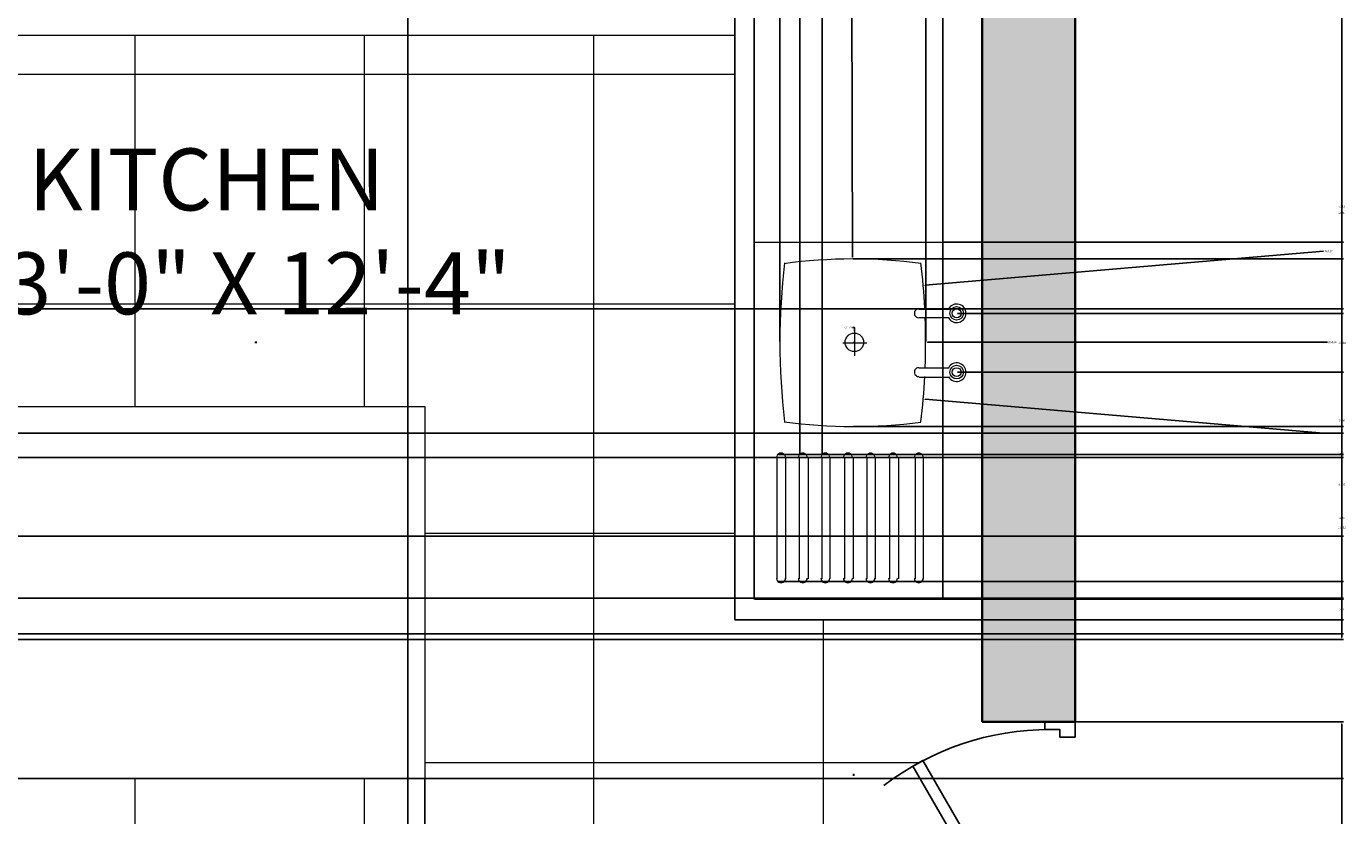
# Model space of a CAD drawing. Units: inches. Extents: x 6 to 575, y 34 to 566.
# Tile 20 of 21: x 447 to 575, y 432 to 508. Entities that reach past the tile are written whole.
import ezdxf

# ---------------------------------------------------------------- set-up
doc = ezdxf.new("R2010")
doc.units = ezdxf.units.IN
for name, color, linetype, lineweight in [('A-ANNO-DIMS', 2, 'Continuous', 18), ('A-AREA-IDEN', 6, 'Continuous', 20), ('A-FLOR-CASE', 2, 'Continuous', 18), ('A-FLOR-FIXT', 9, 'Continuous', 18), ('A-FLOR-PATT', 252, 'Continuous', 9), ('A-WALL-PATT', 251, 'Continuous', 9), ('DOORS', 3, 'Continuous', 25), ('WALLS', 7, 'Continuous', 35)]:
    doc.layers.add(name, color=color, linetype=linetype, lineweight=lineweight)
doc.styles.add('PDF Arial Narrow', font='txt')
doc.styles.get("Standard").update_dxf_attribs({"font": 'arial.ttf'})
doc.dimstyles.get("Standard").update_dxf_attribs({"dimtxt": 0.18, "dimasz": 0.18, "dimexe": 0.18, "dimexo": 0.0625, "dimgap": 0.09, "dimtad": 0, "dimtih": 1, "dimtoh": 1, "dimdec": 4, "dimzin": 0, "dimdsep": 46, "dimtxsty": 'Standard', "dimcen": 0.09, "dimadec": 0, "dimazin": 0, "dimtfac": 1, "dimtdec": 4, "dimtofl": 0, "dimtmove": 0, "dimatfit": 3, "dimfxl": 1, "dimtolj": 1, "dimtzin": 0, "dimarcsym": 0})

# ---------------------------------------------------------------- blocks, each defined once
blk = doc.blocks.new('Door - Left Hung 36 in.')
blk.add_lwpolyline([(0.75, -1.3), (0, 0), (31.18, 18), (31.93, 16.7)], close=True)
blk.add_arc((0, 0), 36, 0, 37.3101)
blk = doc.blocks.new('*D47')
at = {"layer": 'A-ANNO-DIMS', "color": 0, "lineweight": -2, "transparency": 16777216}
for p, q in [((548.72, 440.8), (574.68, 440.8)), ((574.5, 440.62), (574.5, 426.98)), ((574.5, 412.98), (574.5, 426.62)), ((548.72, 412.8), (574.68, 412.8))]:
    blk.add_line(p, q, dxfattribs=at)
at = {"layer": 'A-ANNO-DIMS', "color": 0, "transparency": 16777216}
for points in [[(574.47, 440.62), (574.53, 440.62), (574.5, 440.8)], [(574.47, 412.98), (574.53, 412.98), (574.5, 412.8)]]:
    blk.add_solid(points, dxfattribs=at)
at = {"layer": 'Defpoints', "color": 0, "transparency": 16777216}
for p in [(548.66, 440.8), (574.5, 440.8), (548.66, 412.8)]:
    blk.add_point(p, dxfattribs=at)
at = {"layer": 'A-ANNO-DIMS', "color": 0, "transparency": 16777216, "insert": (574.5, 426.8), "char_height": 0.18, "attachment_point": 5}
blk.add_mtext('\\A1;28', dxfattribs=at)
blk = doc.blocks.new('*D50')
at = {"layer": 'A-ANNO-DIMS', "color": 0, "lineweight": -2, "transparency": 16777216}
for p, q in [((248.7, 468.78), (574.68, 468.78)), ((574.5, 468.6), (574.5, 463.96)), ((574.5, 458.97), (574.5, 463.6)), ((248.7, 458.79), (574.68, 458.79))]:
    blk.add_line(p, q, dxfattribs=at)
at = {"layer": 'A-ANNO-DIMS', "color": 0, "transparency": 16777216}
for points in [[(574.47, 468.6), (574.53, 468.6), (574.5, 468.78)], [(574.47, 458.97), (574.53, 458.97), (574.5, 458.79)]]:
    blk.add_solid(points, dxfattribs=at)
at = {"layer": 'Defpoints', "color": 0, "transparency": 16777216}
for p in [(248.63, 468.78), (574.5, 468.78), (248.63, 458.79)]:
    blk.add_point(p, dxfattribs=at)
at = {"layer": 'A-ANNO-DIMS', "color": 0, "transparency": 16777216, "insert": (574.5, 463.78), "char_height": 0.18, "attachment_point": 5}
blk.add_mtext('\\A1;9.987', dxfattribs=at)
blk = doc.blocks.new('*D51')
at = {"layer": 'A-ANNO-DIMS', "color": 0, "lineweight": -2, "transparency": 16777216}
for p, q in [((437.69, 435.25), (437.69, 33.76)), ((485.67, 435.25), (485.67, 33.76)), ((437.87, 33.94), (461.28, 33.94)), ((485.49, 33.94), (462.08, 33.94))]:
    blk.add_line(p, q, dxfattribs=at)
at = {"layer": 'A-ANNO-DIMS', "color": 0, "transparency": 16777216}
for points in [[(437.87, 33.97), (437.87, 33.91), (437.69, 33.94)], [(485.49, 33.97), (485.49, 33.91), (485.67, 33.94)]]:
    blk.add_solid(points, dxfattribs=at)
at = {"layer": 'Defpoints', "color": 0, "transparency": 16777216}
for p in [(437.69, 435.31), (485.67, 435.31), (485.67, 33.94)]:
    blk.add_point(p, dxfattribs=at)
at = {"layer": 'A-ANNO-DIMS', "color": 0, "transparency": 16777216, "insert": (461.68, 33.94), "char_height": 0.18, "attachment_point": 5}
blk.add_mtext('\\A1;47.98', dxfattribs=at)
blk = doc.blocks.new('*D53')
at = {"layer": 'A-ANNO-DIMS', "color": 0, "lineweight": -2, "transparency": 16777216}
for p, q in [((445.02, 338), (445.02, 565.81)), ((445.2, 565.63), (464.15, 565.63)), ((483.85, 565.63), (464.9, 565.63)), ((484.03, 338), (484.03, 565.81))]:
    blk.add_line(p, q, dxfattribs=at)
at = {"layer": 'A-ANNO-DIMS', "color": 0, "transparency": 16777216}
for points in [[(445.2, 565.66), (445.2, 565.6), (445.02, 565.63)], [(483.85, 565.66), (483.85, 565.6), (484.03, 565.63)]]:
    blk.add_solid(points, dxfattribs=at)
at = {"layer": 'Defpoints', "color": 0, "transparency": 16777216}
for p in [(484.03, 565.63), (445.02, 337.94), (484.03, 337.94)]:
    blk.add_point(p, dxfattribs=at)
at = {"layer": 'A-ANNO-DIMS', "color": 0, "transparency": 16777216, "insert": (464.53, 565.63), "char_height": 0.18, "attachment_point": 5}
blk.add_mtext('\\A1;39.01', dxfattribs=at)
blk = doc.blocks.new('*D64')
at = {"layer": 'A-ANNO-DIMS', "color": 0, "lineweight": -2, "transparency": 16777216}
for p, q in [((354.721145, 452.800984), (574.675816, 452.800984)), ((574.495816, 452.620984), (574.495816, 450.980984)), ((574.495816, 448.980984), (574.495816, 450.620984)), ((354.721145, 448.800984), (574.675816, 448.800984))]:
    blk.add_line(p, q, dxfattribs=at)
at = {"layer": 'A-ANNO-DIMS', "color": 0, "transparency": 16777216}
for points in [[(574.465816, 452.620984), (574.525816, 452.620984), (574.495816, 452.800984)], [(574.465816, 448.980984), (574.525816, 448.980984), (574.495816, 448.800984)]]:
    blk.add_solid(points, dxfattribs=at)
at = {"layer": 'Defpoints', "color": 0, "transparency": 16777216}
for p in [(354.658645, 452.800984), (574.495816, 452.800984), (354.658645, 448.800984)]:
    blk.add_point(p, dxfattribs=at)
at = {"layer": 'A-ANNO-DIMS', "color": 0, "transparency": 16777216, "insert": (574.495816, 450.800984), "char_height": 0.18, "attachment_point": 5}
blk.add_mtext('\\A1;4', dxfattribs=at)
blk = doc.blocks.new('*D151')
at = {"layer": 'A-ANNO-DIMS', "color": 0, "lineweight": -2, "transparency": 16777216}
for p, q in [((437.75, 435.31), (574.68, 435.31)), ((574.5, 435.13), (574.5, 421.25)), ((574.5, 407.01), (574.5, 420.89)), ((433.77, 406.83), (574.68, 406.83))]:
    blk.add_line(p, q, dxfattribs=at)
at = {"layer": 'A-ANNO-DIMS', "color": 0, "transparency": 16777216}
for points in [[(574.47, 435.13), (574.53, 435.13), (574.5, 435.31)], [(574.47, 407.01), (574.53, 407.01), (574.5, 406.83)]]:
    blk.add_solid(points, dxfattribs=at)
at = {"layer": 'Defpoints', "color": 0, "transparency": 16777216}
for p in [(437.69, 435.31), (433.71, 406.83), (574.5, 406.83)]:
    blk.add_point(p, dxfattribs=at)
at = {"layer": 'A-ANNO-DIMS', "color": 0, "transparency": 16777216, "insert": (574.5, 421.07), "char_height": 0.18, "attachment_point": 5}
blk.add_mtext('\\A1;28.48', dxfattribs=at)
blk = doc.blocks.new('*D152')
at = {"layer": 'A-ANNO-DIMS', "color": 0, "lineweight": -2, "transparency": 16777216}
for p, q in [((383.72, 530.8), (574.68, 530.8)), ((574.5, 530.62), (574.5, 490.26)), ((574.5, 449.53), (574.5, 489.89)), ((383.72, 449.35), (574.68, 449.35))]:
    blk.add_line(p, q, dxfattribs=at)
at = {"layer": 'A-ANNO-DIMS', "color": 0, "transparency": 16777216}
for points in [[(574.47, 530.62), (574.53, 530.62), (574.5, 530.8)], [(574.47, 449.53), (574.53, 449.53), (574.5, 449.35)]]:
    blk.add_solid(points, dxfattribs=at)
at = {"layer": 'Defpoints', "color": 0, "transparency": 16777216}
for p in [(383.66, 530.8), (574.5, 530.8), (383.66, 449.35)]:
    blk.add_point(p, dxfattribs=at)
at = {"layer": 'A-ANNO-DIMS', "color": 0, "transparency": 16777216, "insert": (574.5, 490.08), "char_height": 0.18, "attachment_point": 5}
blk.add_mtext('\\A1;81.45', dxfattribs=at)
blk = doc.blocks.new('*D153')
at = {"layer": 'A-ANNO-DIMS', "color": 0, "lineweight": -2, "transparency": 16777216}
for p, q in [((539.72, 530.8), (574.68, 530.8)), ((574.5, 530.62), (574.5, 490.92)), ((574.5, 450.86), (574.5, 490.56)), ((539.72, 450.68), (574.68, 450.68))]:
    blk.add_line(p, q, dxfattribs=at)
at = {"layer": 'A-ANNO-DIMS', "color": 0, "transparency": 16777216}
for points in [[(574.47, 530.62), (574.53, 530.62), (574.5, 530.8)], [(574.47, 450.86), (574.53, 450.86), (574.5, 450.68)]]:
    blk.add_solid(points, dxfattribs=at)
at = {"layer": 'Defpoints', "color": 0, "transparency": 16777216}
for p in [(539.66, 530.8), (574.5, 530.8), (539.66, 450.68)]:
    blk.add_point(p, dxfattribs=at)
at = {"layer": 'A-ANNO-DIMS', "color": 0, "transparency": 16777216, "insert": (574.5, 490.74), "char_height": 0.18, "attachment_point": 5}
blk.add_mtext('\\A1;80.12', dxfattribs=at)
blk = doc.blocks.new('*D155')
at = {"layer": 'A-ANNO-DIMS', "color": 0, "lineweight": -2, "transparency": 16777216}
for p, q in [((515.71, 450.74), (515.71, 565.81)), ((515.89, 565.63), (516.33, 565.63)), ((517.4, 565.63), (516.96, 565.63)), ((517.58, 452.77), (517.58, 565.81))]:
    blk.add_line(p, q, dxfattribs=at)
at = {"layer": 'A-ANNO-DIMS', "color": 0, "transparency": 16777216}
for points in [[(515.89, 565.66), (515.89, 565.6), (515.71, 565.63)], [(517.4, 565.66), (517.4, 565.6), (517.58, 565.63)]]:
    blk.add_solid(points, dxfattribs=at)
at = {"layer": 'Defpoints', "color": 0, "transparency": 16777216}
for p in [(517.58, 565.63), (517.58, 452.71), (515.71, 450.68)]:
    blk.add_point(p, dxfattribs=at)
at = {"layer": 'A-ANNO-DIMS', "color": 0, "transparency": 16777216, "insert": (516.64, 565.63), "char_height": 0.18, "attachment_point": 5}
blk.add_mtext('\\A1;1.87', dxfattribs=at)
blk = doc.blocks.new('*D156')
at = {"layer": 'A-ANNO-DIMS', "color": 0, "lineweight": -2, "transparency": 16777216}
for p, q in [((535.9, 487.27), (574.68, 487.27)), ((574.5, 487.09), (574.5, 470.17)), ((574.5, 452.89), (574.5, 469.81)), ((517.64, 452.71), (574.68, 452.71))]:
    blk.add_line(p, q, dxfattribs=at)
at = {"layer": 'A-ANNO-DIMS', "color": 0, "transparency": 16777216}
for points in [[(574.47, 487.09), (574.53, 487.09), (574.5, 487.27)], [(574.47, 452.89), (574.53, 452.89), (574.5, 452.71)]]:
    blk.add_solid(points, dxfattribs=at)
at = {"layer": 'Defpoints', "color": 0, "transparency": 16777216}
for p in [(535.84, 487.27), (574.5, 487.27), (517.58, 452.71)]:
    blk.add_point(p, dxfattribs=at)
at = {"layer": 'A-ANNO-DIMS', "color": 0, "transparency": 16777216, "insert": (574.5, 469.99), "char_height": 0.18, "attachment_point": 5}
blk.add_mtext('\\A1;34.56', dxfattribs=at)
blk = doc.blocks.new('*D157')
at = {"layer": 'A-ANNO-DIMS', "color": 0, "lineweight": -2, "transparency": 16777216}
for p, q in [((517.58, 452.77), (517.58, 565.81)), ((517.76, 565.63), (526.25, 565.63)), ((535.66, 565.63), (527.16, 565.63)), ((535.84, 452.77), (535.84, 565.81))]:
    blk.add_line(p, q, dxfattribs=at)
at = {"layer": 'A-ANNO-DIMS', "color": 0, "transparency": 16777216}
for points in [[(517.76, 565.66), (517.76, 565.6), (517.58, 565.63)], [(535.66, 565.66), (535.66, 565.6), (535.84, 565.63)]]:
    blk.add_solid(points, dxfattribs=at)
at = {"layer": 'Defpoints', "color": 0, "transparency": 16777216}
for p in [(535.84, 565.63), (517.58, 452.71), (535.84, 452.71)]:
    blk.add_point(p, dxfattribs=at)
at = {"layer": 'A-ANNO-DIMS', "color": 0, "transparency": 16777216, "insert": (526.71, 565.63), "char_height": 0.18, "attachment_point": 5}
blk.add_mtext('\\A1;18.257', dxfattribs=at)
blk = doc.blocks.new('*D158')
at = {"layer": 'A-ANNO-DIMS', "color": 0, "lineweight": -2, "transparency": 16777216}
for p, q in [((517.64, 452.71), (574.68, 452.71)), ((574.5, 452.53), (574.5, 451.87)), ((574.5, 450.86), (574.5, 451.51)), ((515.77, 450.68), (574.68, 450.68))]:
    blk.add_line(p, q, dxfattribs=at)
at = {"layer": 'A-ANNO-DIMS', "color": 0, "transparency": 16777216}
for points in [[(574.47, 452.53), (574.53, 452.53), (574.5, 452.71)], [(574.47, 450.86), (574.53, 450.86), (574.5, 450.68)]]:
    blk.add_solid(points, dxfattribs=at)
at = {"layer": 'Defpoints', "color": 0, "transparency": 16777216}
for p in [(517.58, 452.71), (574.5, 452.71), (515.71, 450.68)]:
    blk.add_point(p, dxfattribs=at)
at = {"layer": 'A-ANNO-DIMS', "color": 0, "transparency": 16777216, "insert": (574.5, 451.69), "char_height": 0.18, "attachment_point": 5}
blk.add_mtext('\\A1;2.03', dxfattribs=at)
blk = doc.blocks.new('*D159')
at = {"layer": 'A-ANNO-DIMS', "color": 0, "lineweight": -2, "transparency": 16777216}
for p, q in [((519.94, 466.72), (574.68, 466.72)), ((574.5, 466.54), (574.5, 460.75)), ((574.5, 454.59), (574.5, 460.38)), ((519.94, 454.41), (574.68, 454.41))]:
    blk.add_line(p, q, dxfattribs=at)
at = {"layer": 'A-ANNO-DIMS', "color": 0, "transparency": 16777216}
for points in [[(574.47, 466.54), (574.53, 466.54), (574.5, 466.72)], [(574.47, 454.59), (574.53, 454.59), (574.5, 454.41)]]:
    blk.add_solid(points, dxfattribs=at)
at = {"layer": 'Defpoints', "color": 0, "transparency": 16777216}
for p in [(519.88, 466.72), (574.5, 466.72), (519.88, 454.41)]:
    blk.add_point(p, dxfattribs=at)
at = {"layer": 'A-ANNO-DIMS', "color": 0, "transparency": 16777216, "insert": (574.5, 460.56), "char_height": 0.18, "attachment_point": 5}
blk.add_mtext('\\A1;12.31', dxfattribs=at)
blk = doc.blocks.new('*D171')
at = {"layer": 'A-ANNO-DIMS', "color": 0, "lineweight": -2, "transparency": 16777216}
for p, q in [((520.07, 477.64), (520.07, 565.81)), ((520.25, 565.63), (526.67, 565.63)), ((534.01, 565.63), (527.58, 565.63)), ((534.19, 477.64), (534.19, 565.81))]:
    blk.add_line(p, q, dxfattribs=at)
at = {"layer": 'A-ANNO-DIMS', "color": 0, "transparency": 16777216}
for points in [[(520.25, 565.66), (520.25, 565.6), (520.07, 565.63)], [(534.01, 565.66), (534.01, 565.6), (534.19, 565.63)]]:
    blk.add_solid(points, dxfattribs=at)
at = {"layer": 'Defpoints', "color": 0, "transparency": 16777216}
for p in [(534.19, 565.63), (520.07, 477.57), (534.19, 477.58)]:
    blk.add_point(p, dxfattribs=at)
at = {"layer": 'A-ANNO-DIMS', "color": 0, "transparency": 16777216, "insert": (527.13, 565.63), "char_height": 0.18, "attachment_point": 5}
blk.add_mtext('\\A1;14.117', dxfattribs=at)
blk = doc.blocks.new('*D172')
at = {"layer": 'A-ANNO-DIMS', "color": 0, "lineweight": -2, "transparency": 16777216}
for p, q in [((527.17, 485.65), (574.68, 485.65)), ((574.5, 485.47), (574.5, 477.72)), ((574.5, 469.6), (574.5, 477.35)), ((527.17, 469.42), (574.68, 469.42))]:
    blk.add_line(p, q, dxfattribs=at)
at = {"layer": 'A-ANNO-DIMS', "color": 0, "transparency": 16777216}
for points in [[(574.47, 485.47), (574.53, 485.47), (574.5, 485.65)], [(574.47, 469.6), (574.53, 469.6), (574.5, 469.42)]]:
    blk.add_solid(points, dxfattribs=at)
at = {"layer": 'Defpoints', "color": 0, "transparency": 16777216}
for p in [(527.1, 485.65), (527.1, 469.42), (574.5, 469.42)]:
    blk.add_point(p, dxfattribs=at)
at = {"layer": 'A-ANNO-DIMS', "color": 0, "transparency": 16777216, "insert": (574.5, 477.53), "char_height": 0.18, "attachment_point": 5}
blk.add_mtext('\\A1;16.224', dxfattribs=at)
blk = doc.blocks.new('*D173')
at = {"layer": 'A-ANNO-DIMS', "color": 0, "lineweight": -2, "transparency": 16777216}
for p, q in [((521.99, 466.78), (521.99, 565.81)), ((522.17, 565.63), (522.75, 565.63)), ((523.99, 565.63), (523.4, 565.63)), ((524.17, 466.78), (524.17, 565.81))]:
    blk.add_line(p, q, dxfattribs=at)
at = {"layer": 'A-ANNO-DIMS', "color": 0, "transparency": 16777216}
for points in [[(522.17, 565.66), (522.17, 565.6), (521.99, 565.63)], [(523.99, 565.66), (523.99, 565.6), (524.17, 565.63)]]:
    blk.add_solid(points, dxfattribs=at)
at = {"layer": 'Defpoints', "color": 0, "transparency": 16777216}
for p in [(524.17, 565.63), (521.99, 466.72), (524.17, 466.72)]:
    blk.add_point(p, dxfattribs=at)
at = {"layer": 'A-ANNO-DIMS', "color": 0, "transparency": 16777216, "insert": (523.08, 565.63), "char_height": 0.18, "attachment_point": 5}
blk.add_mtext('\\A1;2.18', dxfattribs=at)
blk = doc.blocks.new('*D174')
at = {"layer": 'A-ANNO-DIMS', "color": 0, "lineweight": -2, "transparency": 16777216}
for p, q in [((537.26, 480.38), (574.68, 480.38)), ((574.5, 480.2), (574.5, 477.72)), ((574.5, 474.87), (574.5, 477.35)), ((537.26, 474.69), (574.68, 474.69))]:
    blk.add_line(p, q, dxfattribs=at)
at = {"layer": 'A-ANNO-DIMS', "color": 0, "transparency": 16777216}
for points in [[(574.47, 480.2), (574.53, 480.2), (574.5, 480.38)], [(574.47, 474.87), (574.53, 474.87), (574.5, 474.69)]]:
    blk.add_solid(points, dxfattribs=at)
at = {"layer": 'Defpoints', "color": 0, "transparency": 16777216}
for p in [(537.19, 480.38), (574.5, 480.38), (537.19, 474.69)]:
    blk.add_point(p, dxfattribs=at)
at = {"layer": 'A-ANNO-DIMS', "color": 0, "transparency": 16777216, "insert": (574.5, 477.53), "char_height": 0.18, "attachment_point": 5}
blk.add_mtext('\\A1;5.696', dxfattribs=at)
blk = doc.blocks.new('*D194')
at = {"layer": 'A-ANNO-DIMS', "color": 0, "lineweight": -2, "transparency": 16777216}
for p, q in [((374.72, 480.81), (574.68, 480.81)), ((574.5, 480.63), (574.5, 466.99)), ((574.5, 452.98), (574.5, 466.62)), ((356.78, 452.8), (574.68, 452.8))]:
    blk.add_line(p, q, dxfattribs=at)
at = {"layer": 'A-ANNO-DIMS', "color": 0, "transparency": 16777216}
for points in [[(574.47, 480.63), (574.53, 480.63), (574.5, 480.81)], [(574.47, 452.98), (574.53, 452.98), (574.5, 452.8)]]:
    blk.add_solid(points, dxfattribs=at)
at = {"layer": 'Defpoints', "color": 0, "transparency": 16777216}
for p in [(374.66, 480.81), (574.5, 480.81), (356.71, 452.8)]:
    blk.add_point(p, dxfattribs=at)
at = {"layer": 'A-ANNO-DIMS', "color": 0, "transparency": 16777216, "insert": (574.5, 466.81), "char_height": 0.18, "attachment_point": 5}
blk.add_mtext('\\A1;28.01', dxfattribs=at)
blk = doc.blocks.new('*D195')
at = {"layer": 'A-ANNO-DIMS', "color": 0, "lineweight": -2, "transparency": 16777216}
for p, q in [((364.6, 466.43), (574.68, 466.43)), ((574.5, 466.25), (574.5, 459.8)), ((574.5, 452.98), (574.5, 459.44)), ((374.72, 452.8), (574.68, 452.8))]:
    blk.add_line(p, q, dxfattribs=at)
at = {"layer": 'A-ANNO-DIMS', "color": 0, "transparency": 16777216}
for points in [[(574.47, 466.25), (574.53, 466.25), (574.5, 466.43)], [(574.47, 452.98), (574.53, 452.98), (574.5, 452.8)]]:
    blk.add_solid(points, dxfattribs=at)
at = {"layer": 'Defpoints', "color": 0, "transparency": 16777216}
for p in [(364.54, 466.43), (574.5, 466.43), (374.66, 452.8)]:
    blk.add_point(p, dxfattribs=at)
at = {"layer": 'A-ANNO-DIMS', "color": 0, "transparency": 16777216, "insert": (574.5, 459.62), "char_height": 0.18, "attachment_point": 5}
blk.add_mtext('\\A1;13.632', dxfattribs=at)
blk = doc.blocks.new('*D223')
at = {"layer": 'A-ANNO-DIMS', "color": 0, "lineweight": -2, "transparency": 16777216}
for p, q in [((469.22, 477.57), (469.4, 477.57)), ((469.31, 477.48), (469.31, 477.66)), ((573.11, 477.58), (534.37, 477.58))]:
    blk.add_line(p, q, dxfattribs=at)
at = {"layer": 'A-ANNO-DIMS', "color": 0, "transparency": 16777216}
blk.add_solid([(534.37, 477.61), (534.37, 477.55), (534.19, 477.58)], dxfattribs=at)
at = {"layer": 'Defpoints', "color": 0, "transparency": 16777216}
for p in [(469.31, 477.57), (534.19, 477.58)]:
    blk.add_point(p, dxfattribs=at)
at = {"layer": 'A-ANNO-DIMS', "color": 0, "transparency": 16777216, "insert": (573.59, 477.58), "char_height": 0.18, "attachment_point": 5}
blk.add_mtext('\\A1;R64.88', dxfattribs=at)
blk = doc.blocks.new('*D224')
at = {"layer": 'A-ANNO-DIMS', "color": 0, "lineweight": -2, "transparency": 16777216}
for p, q in [((572.74, 486.39), (534.13, 483.1)), ((469.22, 477.57), (469.4, 477.57)), ((469.31, 477.48), (469.31, 477.66))]:
    blk.add_line(p, q, dxfattribs=at)
at = {"layer": 'A-ANNO-DIMS', "color": 0, "transparency": 16777216}
blk.add_solid([(534.13, 483.13), (534.13, 483.07), (533.95, 483.08)], dxfattribs=at)
at = {"layer": 'Defpoints', "color": 0, "transparency": 16777216}
for p in [(533.95, 483.08), (469.31, 477.57)]:
    blk.add_point(p, dxfattribs=at)
at = {"layer": 'A-ANNO-DIMS', "color": 0, "transparency": 16777216, "insert": (573.22, 486.39), "char_height": 0.18, "attachment_point": 5}
blk.add_mtext('\\A1;R64.87', dxfattribs=at)
blk = doc.blocks.new('*D225')
at = {"layer": 'A-ANNO-DIMS', "color": 0, "lineweight": -2, "transparency": 16777216}
for p, q in [((469.23, 477.57), (469.41, 477.57)), ((469.32, 477.48), (469.32, 477.66)), ((572.73, 468.77), (534.13, 472.06))]:
    blk.add_line(p, q, dxfattribs=at)
at = {"layer": 'A-ANNO-DIMS', "color": 0, "transparency": 16777216}
blk.add_solid([(534.13, 472.09), (534.13, 472.03), (533.95, 472.07)], dxfattribs=at)
at = {"layer": 'Defpoints', "color": 0, "transparency": 16777216}
for p in [(469.32, 477.57), (533.95, 472.07)]:
    blk.add_point(p, dxfattribs=at)
at = {"layer": 'A-ANNO-DIMS', "color": 0, "transparency": 16777216, "insert": (573.21, 468.77), "char_height": 0.18, "attachment_point": 5}
blk.add_mtext('\\A1;R64.87', dxfattribs=at)
blk = doc.blocks.new('*D227')
at = {"layer": 'A-ANNO-DIMS', "color": 0, "lineweight": -2, "transparency": 16777216}
for p, q in [((526.86, 515.63), (527.04, 515.63)), ((527.04, 515.63), (527.1, 485.83)), ((527.12, 435.68), (527.3, 435.68)), ((527.21, 435.59), (527.21, 435.77))]:
    blk.add_line(p, q, dxfattribs=at)
at = {"layer": 'A-ANNO-DIMS', "color": 0, "transparency": 16777216}
blk.add_solid([(527.13, 485.83), (527.07, 485.83), (527.1, 485.65)], dxfattribs=at)
at = {"layer": 'Defpoints', "color": 0, "transparency": 16777216}
for p in [(527.1, 485.65), (527.21, 435.68)]:
    blk.add_point(p, dxfattribs=at)
at = {"layer": 'A-ANNO-DIMS', "color": 0, "transparency": 16777216, "insert": (526.19, 515.63), "char_height": 0.18, "attachment_point": 5}
blk.add_mtext('\\A1;2X R49.97', dxfattribs=at)
blk = doc.blocks.new('*D250')
at = {"layer": 'A-ANNO-DIMS', "color": 0, "lineweight": -2, "transparency": 16777216}
for p, q in [((527.1, 479.01), (527.28, 479.01)), ((527.28, 479.01), (527.28, 478.65)), ((527.19, 477.57), (527.37, 477.57)), ((527.28, 477.48), (527.28, 477.66))]:
    blk.add_line(p, q, dxfattribs=at)
at = {"layer": 'A-ANNO-DIMS', "color": 0, "transparency": 16777216}
blk.add_solid([(527.31, 478.65), (527.25, 478.65), (527.28, 478.47)], dxfattribs=at)
at = {"layer": 'Defpoints', "color": 0, "transparency": 16777216}
for p in [(527.28, 478.47), (527.29, 476.68)]:
    blk.add_point(p, dxfattribs=at)
at = {"layer": 'A-ANNO-DIMS', "color": 0, "transparency": 16777216, "insert": (526.68, 479.01), "char_height": 0.18, "attachment_point": 5}
blk.add_mtext('\\A1;∅1.79', dxfattribs=at)

msp = doc.modelspace()

# ---------------------------------------------------------------- hatches: boundary and pattern name
at = {"layer": 'A-FLOR-PATT'}
h = msp.add_hatch(dxfattribs=at)
h.set_pattern_fill('NET', color=256, scale=7)
h.set_pattern_definition([(0, (-98.035, 170.147), (0, 22.225), []), (90, (-98.035, 170.147), (-22.225, 1e-15), [])])
h.paths.add_polyline_path([(539.6586, 366.801), (539.6586, 378.801), (433.708, 378.801), (383.6586, 378.801), (383.6586, 278.801), (383.6586, 224.801), (383.6586, 212.801), (407.6586, 212.801), (515.6586, 212.801), (539.6586, 212.801), (539.6586, 270.801)])
h.paths.add_polyline_path([(434.8003, 333.3365), (436.6727, 333.3365), (436.6727, 331.9322), (445.0208, 331.9322), (445.0208, 337.9397), (456.1776, 337.9397), (456.1776, 346.2878), (454.7733, 346.2878), (454.7733, 348.1603), (474.2782, 348.1603), (474.2782, 346.2878), (472.8738, 346.2878), (472.8738, 337.9397), (484.0307, 337.9397), (484.0307, 331.9322), (492.3788, 331.9322), (492.3788, 333.3365), (494.2512, 333.3365), (494.2512, 313.8316), (492.3788, 313.8316), (492.3788, 315.158), (484.0307, 315.158), (484.0307, 307.278), (492.3788, 307.278), (492.3788, 308.6823), (494.2512, 308.6823), (494.2512, 289.1774), (492.3788, 289.1774), (492.3788, 290.5818), (484.0307, 290.5818), (484.0307, 282.7018), (492.3788, 282.7018), (492.3788, 284.1062), (494.2512, 284.1062), (494.2512, 264.6013), (492.3788, 264.6013), (492.3788, 266.0056), (484.0307, 266.0056), (484.0307, 259.9201), (472.8738, 259.9201), (472.8738, 251.572), (474.2782, 251.572), (474.2782, 249.6995), (454.7733, 249.6995), (454.7733, 251.572), (456.1776, 251.572), (456.1776, 259.9201), (445.0208, 259.9201), (445.0208, 266.0056), (436.6727, 266.0056), (436.6727, 264.6013), (434.8003, 264.6013), (434.8003, 284.1062), (436.6727, 284.1062), (436.6727, 282.7018), (445.0208, 282.7018), (445.0208, 290.5818), (436.6727, 290.5818), (436.6727, 289.1774), (434.8003, 289.1774), (434.8003, 308.6823), (436.6727, 308.6823), (436.6727, 307.278), (445.0208, 307.278), (445.0208, 315.158), (436.6727, 315.158), (436.6727, 313.8316), (434.8003, 313.8316)], flags=16)
h.paths.add_polyline_path([(532.9619, 436.5144), (533.9192, 437.0672), (533.9307, 437.0472, -0.12106636), (546.2274, 440.0689), (539.6586, 440.801), (539.6586, 450.6781), (515.7066, 450.6781), (515.7066, 507.3203), (407.6494, 507.3203), (407.6494, 449.3517), (383.6586, 449.3517), (383.6586, 382.801), (433.708, 382.801), (433.708, 406.831), (539.6586, 406.831), (539.6586, 412.801), (545.7108, 412.801), (545.7108, 414.4327)])
h.paths.add_polyline_path([(437.687, 435.3082), (437.687, 471.3533), (485.6691, 471.3533), (485.6691, 435.3082)], flags=16)
at = {"layer": 'A-WALL-PATT'}
h = msp.add_hatch(color=256, dxfattribs=at)
h.dxf.hatch_style = 1
h.paths.add_polyline_path([(160.6586, 539.801), (32.6586, 539.801), (32.6586, 272.801), (41.6586, 272.801), (41.6586, 286.0643), (41.6586, 358.0764), (41.6586, 379.0637), (41.6586, 407.7709), (41.6194, 407.7709), (41.6194, 431.801), (82.8918, 431.801), (82.8918, 440.801), (65.6494, 440.801), (65.6494, 440.7732), (41.6194, 440.7732), (41.6194, 515.5941), (41.6586, 530.801), (117.6586, 530.801), (117.6586, 474.801), (120.6068, 474.801), (121.6586, 474.801), (121.6586, 530.801), (137.4275, 530.801), (137.4275, 530.8356), (141.2505, 530.8356), (160.6586, 530.801)])
h.paths.add_polyline_path([(71.6586, 212.801), (41.6586, 212.801), (41.6586, 224.801), (32.6586, 224.801), (32.6586, 203.801), (71.6586, 203.801)])
h.paths.add_polyline_path([(206.6586, 215.801), (246.6586, 215.801), (246.6586, 224.801), (206.6586, 224.801), (206.6586, 230.801), (201.8157, 230.801), (197.6586, 230.801), (197.6586, 212.801), (167.6586, 212.801), (167.6586, 203.801), (206.6586, 203.801)])
h.paths.add_polyline_path([(383.6586, 224.801), (334.6586, 224.801), (334.6586, 215.801), (374.6586, 215.801), (374.6586, 203.801), (384.0753, 203.801), (407.6586, 203.801), (407.6586, 212.801), (383.6586, 212.801)])
h.paths.add_polyline_path([(548.6586, 270.801), (539.6586, 270.801), (539.6586, 212.801), (515.6586, 212.801), (515.6586, 203.801), (548.6586, 203.801)])
h.paths.add_polyline_path([(548.6586, 412.801), (545.7108, 412.801), (539.6586, 412.801), (539.6586, 382.801), (433.708, 382.801), (433.708, 378.801), (539.6586, 378.801), (539.6586, 366.801), (548.6586, 366.801)])
h.paths.add_polyline_path([(548.6586, 539.801), (455.9436, 539.801), (455.9436, 530.801), (539.6586, 530.801), (539.6586, 440.801), (548.6586, 440.801)])
h.paths.add_polyline_path([(407.9436, 539.801), (362.6586, 539.801), (362.6586, 530.801), (374.6586, 530.801), (374.6586, 452.801), (354.6586, 452.801), (354.6586, 448.801), (374.6586, 448.801), (374.6586, 278.801), (383.6586, 278.801), (383.6586, 530.801), (407.9436, 530.801)])
h.paths.add_polyline_path([(338.6586, 539.801), (320.6586, 539.801), (320.6586, 530.801), (322.6586, 530.801), (322.6586, 448.801), (326.6586, 448.801), (326.6586, 530.801), (338.6586, 530.801)])
h.paths.add_polyline_path([(272.6586, 539.801), (184.6586, 539.801), (184.6586, 530.801), (197.6586, 530.801), (197.6586, 440.801), (176.6714, 440.801), (121.6586, 440.801), (121.6586, 446.801), (117.6586, 446.801), (117.6586, 440.801), (111.6586, 440.801), (111.6586, 431.801), (197.6586, 431.801), (197.6586, 407.7709), (197.6586, 276.801), (206.6586, 276.801), (206.6586, 530.801), (272.6586, 530.801)])

# ---------------------------------------------------------------- linework, layer by layer
at = {"layer": 'A-FLOR-CASE'}
msp.add_lwpolyline([(383.6586, 449.3517), (407.6494, 449.3517), (407.6494, 507.3203), (515.7066, 507.3203), (515.7066, 450.6781), (539.6586, 450.6781)], dxfattribs=at)
msp.add_lwpolyline([(437.687, 471.3533), (485.6691, 471.3533), (485.6691, 435.3082), (437.687, 435.3082)], close=True, dxfattribs=at)
at = {"layer": 'A-FLOR-FIXT'}
for points in [[(535.8357, 474.162), (535.8357, 452.7066), (517.5791, 452.7066), (517.5791, 487.2693), (535.8357, 487.2693), (535.8357, 480.7936)], [(533.5731, 480.7936), (536.4598, 480.7936)], [(536.4598, 479.9354), (533.5731, 479.9354)], [(535.8357, 479.9354), (535.8357, 475.0982)], [(527.3315, 476.2685), (527.3315, 478.7651)], [(526.1612, 477.5168), (528.5018, 477.5168)], [(533.5731, 475.0982), (536.4598, 475.0982)], [(536.4598, 474.162), (533.5731, 474.162)], [(519.7636, 466.36), (519.7636, 454.6571)], [(520.6219, 466.36), (520.6219, 454.6571)], [(521.9482, 466.36), (521.9482, 454.6571)], [(522.8064, 466.36), (522.8064, 454.6571)], [(524.1327, 466.36), (524.1327, 454.6571)], [(524.9129, 466.36), (524.9129, 454.6571)], [(526.3173, 466.36), (526.3173, 454.6571)], [(527.1755, 466.36), (527.1755, 454.6571)], [(528.5018, 466.36), (528.5018, 454.6571)], [(529.282, 466.36), (529.282, 454.6571)], [(530.6864, 466.36), (530.6864, 454.6571)], [(531.5446, 466.36), (531.5446, 454.6571)], [(533.183, 466.36), (533.183, 454.6571)], [(533.9632, 466.36), (533.9632, 454.6571)]]:
    msp.add_lwpolyline(points, dxfattribs=at)
for centre, radius in [((537.1925, 480.3827), 0.6632), ((537.1925, 480.3827), 0.4291), ((527.2836, 477.5739), 0.8972), ((537.1925, 474.687), 0.6632), ((537.1925, 474.687), 0.4291)]:
    msp.add_circle(centre, radius, dxfattribs=at)
for centre, radius, start, end in [((527.2056, 435.6757), 49.9715, 82.49083, 97.745373), ((584.9424, 477.5739), 64.8732, 173.193956, 186.806044), ((469.3117, 477.5738), 64.8744, 2.933398, 6.806015), ((533.5255, 480.3827), 0.4291, 89.999948, 270.000052), ((537.1925, 480.3827), 0.8972, 210.245407, 149.655749), ((469.3101, 477.5739), 64.8759, 357.885238, 2.125789), ((537.1925, 474.687), 0.8972, 210.245407, 149.655749), ((533.5255, 474.687), 0.4291, 89.999948, 270.000052), ((469.316, 477.5736), 64.8701, 353.193883, 357.077745), ((527.2056, 519.394), 49.9715, 262.254627, 277.50917), ((520.1836, 466.4166), 0.4291, 0, 180.000052), ((522.2902, 466.4166), 0.4291, 0, 180.000052), ((524.4748, 466.4166), 0.4291, 0, 180.000052), ((526.6595, 466.4166), 0.4291, 0, 180.000052), ((528.8441, 466.4166), 0.4291, 0, 180.000052), ((531.0287, 466.4166), 0.4291, 0, 180.000052), ((533.5255, 466.4166), 0.4291, 0, 180.000052), ((520.1836, 454.7132), 0.4291, 179.999948, 359.999948), ((522.2902, 454.7132), 0.4291, 179.999948, 359.999948), ((524.4748, 454.7132), 0.4291, 179.999948, 359.999948), ((526.6595, 454.7132), 0.4291, 179.999948, 359.999948), ((528.8441, 454.7132), 0.4291, 179.999948, 359.999948), ((531.0287, 454.7132), 0.4291, 179.999948, 359.999948), ((533.5255, 454.7132), 0.4291, 179.999948, 359.999948)]:
    msp.add_arc(centre, radius, start, end, dxfattribs=at)
at = {"layer": 'DOORS'}
msp.add_lwpolyline([(548.6658, 439.327), (548.6658, 440.801), (545.7179, 440.801), (545.7179, 440.064), (547.1919, 440.064), (547.1919, 439.327)], close=True, dxfattribs=at)
at = {"layer": 'WALLS'}
for p, q in [((548.6586, 539.801), (548.6586, 440.801)), ((539.6586, 530.801), (539.6586, 440.801)), ((539.6586, 440.801), (548.6586, 440.801))]:
    msp.add_line(p, q, dxfattribs=at)

# ---------------------------------------------------------------- block references
at = {"layer": 'DOORS', "xscale": 0.7369707940286819, "yscale": 0.7369707940286819, "zscale": 0.7369707940286819, "rotation": 90.00000000000003}
msp.add_blockref('Door - Left Hung 36 in.', (546.2274, 413.538), dxfattribs=at)

# ---------------------------------------------------------------- texts
at = {"layer": 'A-AREA-IDEN', "attachment_point": 4, "style": 'PDF Arial Narrow'}
for s, insert, char_height in [('KITCHEN', (447.2663, 492.5691), 6.0005), ('13\'-0" X 12\'-4"', (440.4003, 482.5041), 6.000503)]:
    msp.add_mtext(s, dxfattribs=dict(at, insert=insert, char_height=char_height))

# ---------------------------------------------------------------- dimensions: what is measured, and where the dimension line sits
at = {"layer": 'A-ANNO-DIMS'}
for base, p1, p2, override, picture, middle in [((484.0307, 565.631), (445.0208, 337.9397), (484.0307, 337.9397), {"dimdec": 2, "dimlfac": 1, "dimrnd": 0, "dimzin": 0, "dimdsep": 46, "dimlunit": 2}, '*D53', (464.5257, 565.631)), ((517.5791, 565.631), (515.7066, 450.6781), (517.5791, 452.7066), {"dimdec": 2, "dimlfac": 1, "dimrnd": 0, "dimzin": 0, "dimdsep": 46, "dimlunit": 2}, '*D155', (516.6429, 565.631)), ((535.8357, 565.631), (517.5791, 452.7066), (535.8357, 452.7066), {"dimdec": 3, "dimlfac": 1, "dimrnd": 0, "dimzin": 0, "dimdsep": 46, "dimlunit": 2}, '*D157', (526.7074, 565.631)), ((534.186, 565.631), (520.0692, 477.5739), (534.186, 477.5801), {"dimdec": 3, "dimlfac": 1, "dimrnd": 0, "dimzin": 0, "dimdsep": 46, "dimlunit": 2}, '*D171', (527.1276, 565.631)), ((524.1707, 565.631), (521.9861, 466.7194), (524.1707, 466.7194), {"dimdec": 2, "dimlfac": 1, "dimrnd": 0, "dimzin": 0, "dimdsep": 46, "dimlunit": 2}, '*D173', (523.0784, 565.631)), ((485.6691, 33.9447), (437.687, 435.3082), (485.6691, 435.3082), {"dimdec": 2, "dimlfac": 1, "dimrnd": 0, "dimzin": 0, "dimdsep": 46, "dimlunit": 2}, '*D51', (461.678, 33.9447))]:
    dim = msp.add_linear_dim(base=base, p1=p1, p2=p2, dimstyle='Standard', override=override, dxfattribs=at)
    dim.commit()
    dim.dimension.update_dxf_attribs({"geometry": picture, "text_midpoint": middle})
for base, p1, p2, override, picture, middle in [((574.4958, 530.801), (383.6586, 449.3517), (383.6586, 530.801), {"dimdec": 2, "dimlfac": 1, "dimrnd": 0, "dimzin": 0, "dimdsep": 46, "dimlunit": 2}, '*D152', (574.4958, 490.0764)), ((574.4958, 530.801), (539.6586, 450.6781), (539.6586, 530.801), {"dimdec": 2, "dimlfac": 1, "dimrnd": 0, "dimzin": 0, "dimdsep": 46, "dimlunit": 2}, '*D153', (574.4958, 490.7395)), ((574.4958, 487.2693), (517.5791, 452.7066), (535.8357, 487.2693), {"dimdec": 2, "dimlfac": 1, "dimrnd": 0, "dimzin": 0, "dimdsep": 46, "dimlunit": 2}, '*D156', (574.4958, 469.9879)), ((574.49582, 469.42264), (527.10262, 485.6471), (527.10262, 469.42264), {"dimdec": 3, "dimlfac": 1, "dimrnd": 0, "dimzin": 0, "dimdsep": 46, "dimlunit": 2}, '*D172', (574.49582, 477.53487)), ((574.4958, 480.81), (356.7141, 452.801), (374.6586, 480.81), {"dimdec": 2, "dimlfac": 1, "dimrnd": 0, "dimzin": 0, "dimdsep": 46, "dimlunit": 2}, '*D194', (574.4958, 466.8055)), ((574.4958, 480.3827), (537.1925, 474.687), (537.1925, 480.3827), {"dimdec": 3, "dimlfac": 1, "dimrnd": 0, "dimzin": 0, "dimdsep": 46, "dimlunit": 2}, '*D174', (574.4958, 477.5349)), ((574.49582, 468.77538), (248.6332, 458.78887), (248.6332, 468.77538), {"dimdec": 3, "dimlfac": 1, "dimrnd": 0, "dimzin": 0, "dimdsep": 46, "dimlunit": 2}, '*D50', (574.49582, 463.78213)), ((574.4958, 466.7194), (519.8795, 454.4104), (519.8795, 466.7194), {"dimdec": 2, "dimlfac": 1, "dimrnd": 0, "dimzin": 0, "dimdsep": 46, "dimlunit": 2}, '*D159', (574.4958, 460.5649)), ((574.4958, 466.433), (374.6586, 452.801), (364.5396, 466.433), {"dimdec": 3, "dimlfac": 1, "dimrnd": 0, "dimzin": 0, "dimdsep": 46, "dimlunit": 2}, '*D195', (574.4958, 459.617)), ((574.4958, 452.801), (354.6586, 448.801), (354.6586, 452.801), {"dimdec": 0, "dimlfac": 1, "dimrnd": 0, "dimzin": 0, "dimdsep": 46, "dimlunit": 2}, '*D64', (574.4958, 450.801)), ((574.4958, 452.7066), (515.7066, 450.6781), (517.5791, 452.7066), {"dimdec": 2, "dimlfac": 1, "dimrnd": 0, "dimzin": 0, "dimdsep": 46, "dimlunit": 2}, '*D158', (574.4958, 451.6923)), ((574.4958, 440.801), (548.6586, 412.801), (548.6586, 440.801), {"dimdec": 0, "dimlfac": 1, "dimrnd": 0, "dimzin": 0, "dimdsep": 46, "dimlunit": 2}, '*D47', (574.4958, 426.801)), ((574.4958, 406.831), (437.687, 435.3082), (433.708, 406.831), {"dimdec": 2, "dimlfac": 1, "dimrnd": 0, "dimzin": 0, "dimdsep": 46, "dimlunit": 2}, '*D151', (574.4958, 421.0696))]:
    dim = msp.add_linear_dim(base=base, p1=p1, p2=p2, angle=90, dimstyle='Standard', override=override, dxfattribs=at)
    dim.commit()
    dim.dimension.update_dxf_attribs({"geometry": picture, "text_midpoint": middle})
dim = msp.add_radius_dim(center=(527.2056, 435.6757), mpoint=(527.103, 485.6471), text='2X <>', dimstyle='Standard', override={"dimdec": 2, "dimlfac": 1, "dimrnd": 0, "dimzin": 0, "dimdsep": 46, "dimlunit": 2}, dxfattribs=at)
dim.commit()
dim.dimension.update_dxf_attribs({"geometry": '*D227', "text_midpoint": (526.1867, 515.6299), "dimtype": 164})
for center, mpoint, picture, middle in [((469.3117, 477.5738), (533.9519, 483.081), '*D224', (572.736, 486.3853)), ((469.3101, 477.5739), (534.186, 477.58), '*D223', (573.1116, 477.5837)), ((469.316, 477.5736), (533.9524, 472.073), '*D225', (572.7343, 468.7726))]:
    dim = msp.add_radius_dim(center=center, mpoint=mpoint, dimstyle='Standard', override={"dimdec": 2, "dimlfac": 1, "dimrnd": 0, "dimzin": 0, "dimdsep": 46, "dimlunit": 2}, dxfattribs=at)
    dim.commit()
    dim.dimension.update_dxf_attribs({"geometry": picture, "text_midpoint": middle, "dimtype": 164})
dim = msp.add_diameter_dim_2p(p1=(527.2873, 476.6767), p2=(527.28, 478.4711), dimstyle='Standard', override={"dimdec": 2, "dimlfac": 1, "dimrnd": 0, "dimzin": 0, "dimdsep": 46, "dimlunit": 2}, dxfattribs=at)
dim.commit()
dim.dimension.update_dxf_attribs({"geometry": '*D250', "text_midpoint": (526.676, 479.0094), "dimtype": 163})

doc.saveas('drawing.dxf')
